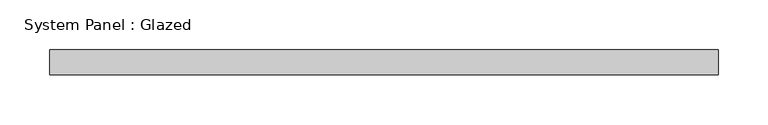
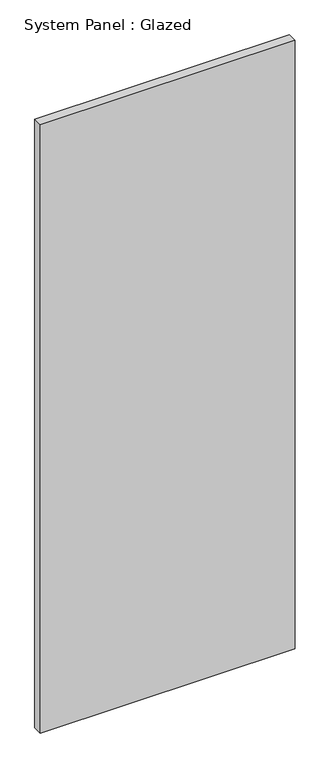
"""IFC4 building model written with IfcOpenShell, lengths in millimetres: plate geometry, System Panel : Glazed."""

from ifc_helpers import new_model, si_unit, origin, origin_with_axes, place, context, project, spatial, polyline, outline, extrude, source, transform, mapped, element, save


def system_panel_glazed_980f9714(model_context):
    return source(origin(), model_context, "Body", "SweptSolid", [
        extrude(outline(polyline([(337.2685902, 19.05), (-337.2685902, 19.05), (-337.2685902, 44.45), (337.2685902, 44.45), (337.2685902, 19.05)])), origin_with_axes(), (0.0, 0.0, 1.0), 1703.5048712),
    ])


if __name__ == "__main__":
    model = new_model("IFC4")
    model_context = context("Model", 3, world=origin())
    ifc_project = project(units=[si_unit("LENGTHUNIT", "METRE", prefix="MILLI")], contexts=[model_context])
    site = spatial("IfcSite", under=ifc_project)
    building = spatial("IfcBuilding", under=site)
    placement = place(None, origin())
    system_panel_glazed_shape = system_panel_glazed_980f9714(model_context)
    element("IfcPlate", 1, ObjectType="System Panel : Glazed", at=placement, inside=building, context=model_context, shape_type="MappedRepresentation", body=[
        mapped(system_panel_glazed_shape, transform((0.0, 0.0, 0.0), x_axis=(1.0, 0.0, 0.0), y_axis=(0.0, 1.0, 0.0), z_axis=(0.0, 0.0, 1.0))),
    ])
    save(model, "model.ifc")

# Revit data of these elements
# Type "System Panel : Glazed"
#   Construction Type Id = "GSP4R"
#   Analytic Construction = "1/8 in Pilkington single glazing"
#   Visual Light Transmittance = 0.9
#   Solar Heat Gain Coefficient = 0.86
#   Heat Transfer Coefficient (U) = 1.18115 BTU/(h·ft²·°F)
#   Define Thermal Properties by = 1
# Element 1 (IfcPlate, "System Panel : Glazed")
#   Materials on its faces: "Glass"
# Materials
#   "Glass": class "Glass", colour RGB 0 128 192, transparency 0.75, Description = "Soda Lime Glass", Cost = 0
